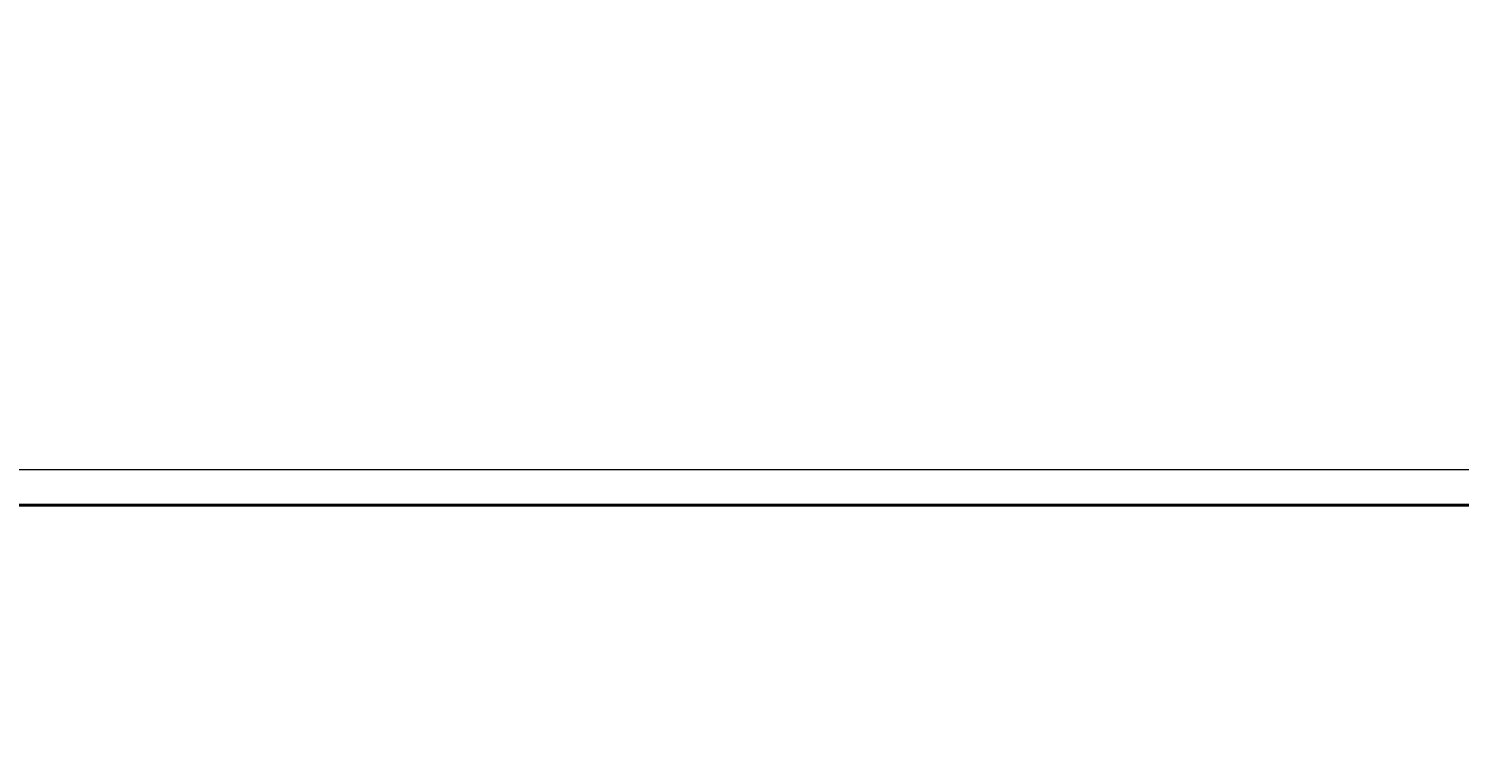
# Model space of a CAD drawing. Units: inches. Extents: x -301 to 715, y -607 to 364.
# Tile 78 of 141: x -94 to -61, y -73 to -56. Entities that reach past the tile are written whole.
import ezdxf

# ---------------------------------------------------------------- set-up
doc = ezdxf.new("R2010")
doc.units = ezdxf.units.IN
doc.header["$MEASUREMENT"] = 0
for name, color, linetype, lineweight in [('A-ANNO-DIMS', 2, 'Continuous', 18), ('A-FURN', 8, 'Continuous', 18), ('A-WALL', 3, 'Continuous', 40)]:
    doc.layers.add(name, color=color, linetype=linetype, lineweight=lineweight)
doc.styles.get("Standard").update_dxf_attribs({"font": 'arial.ttf'})
doc.dimstyles.get("Standard").update_dxf_attribs({"dimtxt": 0.18, "dimasz": 0.18, "dimexe": 0.18, "dimexo": 0.0625, "dimgap": 0.09, "dimtad": 0, "dimtih": 1, "dimtoh": 1, "dimdec": 1, "dimzin": 0, "dimdsep": 46, "dimlunit": 4, "dimtxsty": 'Standard', "dimcen": 0.09, "dimclrd": 3, "dimclre": 4, "dimclrt": 6, "dimadec": 0, "dimazin": 0, "dimtfac": 1, "dimtdec": 1, "dimtofl": 0, "dimtmove": 0, "dimatfit": 3, "dimfxl": 1, "dimtfill": 2, "dimtfillclr": 51, "dimtolj": 1, "dimtzin": 0, "dimarcsym": 0})

# ---------------------------------------------------------------- blocks, each defined once
blk = doc.blocks.new('Desk - 30 x 60 in.')
blk.add_line((-26.999995, 0), (26.999995, 0))
blk = doc.blocks.new('*D57')
at = {"layer": 'A-ANNO-DIMS', "color": 0, "lineweight": -2, "transparency": 16777216}
for p, q in [((-195.603, -67.255), (-195.603, -42.99)), ((-190.603, -43.17), (-126.098, -43.17)), ((-56.603, -43.17), (-121.109, -43.17)), ((-51.603, -67.255), (-51.603, -42.99))]:
    blk.add_line(p, q, dxfattribs=at)
at = {"layer": 'A-ANNO-DIMS', "color": 0, "transparency": 16777216}
for points in [[(-190.603, -42.336), (-190.603, -44.003), (-195.603, -43.17)], [(-56.603, -42.336), (-56.603, -44.003), (-51.603, -43.17)]]:
    blk.add_solid(points, dxfattribs=at)
at = {"layer": 'Defpoints', "color": 0, "transparency": 16777216}
for p in [(-51.603, -43.17), (-195.603, -67.318), (-51.603, -67.318)]:
    blk.add_point(p, dxfattribs=at)
at = {"layer": 'A-ANNO-DIMS', "color": 0, "transparency": 16777216, "insert": (-123.603, -43.17), "char_height": 3, "attachment_point": 5, "bg_fill": 1, "box_fill_scale": 1.25, "bg_fill_color": 51, "bg_fill_transparency": 0}
blk.add_mtext("\\A1;12'", dxfattribs=at)
blk = doc.blocks.new('*D151')
at = {"layer": 'A-ANNO-DIMS', "color": 4, "lineweight": -2, "transparency": 16777216}
for p, q in [((-204.603, -223.755), (-204.603, 359.612)), ((-45.603, -214.755), (-45.603, 359.612))]:
    blk.add_line(p, q, dxfattribs=at)
at = {"layer": 'A-ANNO-DIMS', "color": 3, "lineweight": -2, "transparency": 16777216}
for p, q in [((-204.423, 359.432), (-125.494, 359.432)), ((-45.783, 359.432), (-124.713, 359.432))]:
    blk.add_line(p, q, dxfattribs=at)
at = {"layer": 'A-ANNO-DIMS', "color": 3, "transparency": 16777216}
for points in [[(-204.423, 359.462), (-204.423, 359.402), (-204.603, 359.432)], [(-45.783, 359.462), (-45.783, 359.402), (-45.603, 359.432)]]:
    blk.add_solid(points, dxfattribs=at)
at = {"layer": 'Defpoints', "color": 0, "transparency": 16777216}
for p in [(-45.603, 359.432), (-45.603, -214.818), (-204.603, -223.818)]:
    blk.add_point(p, dxfattribs=at)
at = {"layer": 'A-ANNO-DIMS', "color": 6, "transparency": 16777216, "insert": (-125.103, 359.432), "char_height": 0.18, "attachment_point": 5, "bg_fill": 1, "box_fill_scale": 1.25, "bg_fill_color": 51, "bg_fill_transparency": 0}
blk.add_mtext('\\A1;13\'-3"', dxfattribs=at)
blk = doc.blocks.new('*D158')
at = {"layer": 'A-ANNO-DIMS', "color": 4, "lineweight": -2, "transparency": 16777216}
for p, q in [((-122.603, 221.62), (-122.603, -296.865)), ((-50.603, 221.62), (-50.603, -296.865))]:
    blk.add_line(p, q, dxfattribs=at)
at = {"layer": 'A-ANNO-DIMS', "color": 3, "lineweight": -2, "transparency": 16777216}
for p, q in [((-122.423, -296.685), (-86.933, -296.685)), ((-50.783, -296.685), (-86.274, -296.685))]:
    blk.add_line(p, q, dxfattribs=at)
at = {"layer": 'A-ANNO-DIMS', "color": 3, "transparency": 16777216}
for points in [[(-122.423, -296.655), (-122.423, -296.715), (-122.603, -296.685)], [(-50.783, -296.655), (-50.783, -296.715), (-50.603, -296.685)]]:
    blk.add_solid(points, dxfattribs=at)
at = {"layer": 'Defpoints', "color": 0, "transparency": 16777216}
for p in [(-122.603, 221.682), (-50.603, 221.682), (-50.603, -296.685)]:
    blk.add_point(p, dxfattribs=at)
at = {"layer": 'A-ANNO-DIMS', "color": 6, "transparency": 16777216, "insert": (-86.603, -296.685), "char_height": 0.18, "attachment_point": 5, "bg_fill": 1, "box_fill_scale": 1.25, "bg_fill_color": 51, "bg_fill_transparency": 0}
blk.add_mtext('\\A1;6\'-0"', dxfattribs=at)

msp = doc.modelspace()

# ---------------------------------------------------------------- linework, layer by layer
at = {"layer": 'A-WALL'}
msp.add_line((-195.603, -67.318), (-51.603, -67.318), dxfattribs=at)

# ---------------------------------------------------------------- block references
at = {"layer": 'A-FURN', "xscale": -0.8558048107780498, "yscale": 0.8558048107780498, "zscale": 0.8558048107780498, "rotation": 180}
msp.add_blockref('Desk - 30 x 60 in.', (-77.803, -66.488), dxfattribs=at)

# ---------------------------------------------------------------- dimensions: what is measured, and where the dimension line sits
at = {"layer": 'A-ANNO-DIMS'}
for base, p1, p2, override, picture, middle in [((-45.603, 359.432), (-204.603, -223.818), (-45.603, -214.818), {"dimdec": 1, "dimlfac": 1, "dimrnd": 0, "dimzin": 1, "dimdsep": 46, "dimlunit": 4, "dimfrac": 2}, '*D151', (-125.103, 359.432)), ((-50.603, -296.685), (-122.603, 221.682), (-50.603, 221.682), {"dimdec": 1, "dimlfac": 1, "dimrnd": 0, "dimzin": 1, "dimdsep": 46, "dimlunit": 4, "dimfrac": 2}, '*D158', (-86.603, -296.685)), ((-51.603, -43.17), (-195.603, -67.318), (-51.603, -67.318), {"dimtxt": 3, "dimasz": 5, "dimclrd": 0, "dimclre": 0, "dimclrt": 0}, '*D57', (-123.603, -43.17))]:
    dim = msp.add_linear_dim(base=base, p1=p1, p2=p2, dimstyle='Standard', override=override, dxfattribs=at)
    dim.commit()
    dim.dimension.update_dxf_attribs({"geometry": picture, "text_midpoint": middle})

doc.saveas('drawing.dxf')
